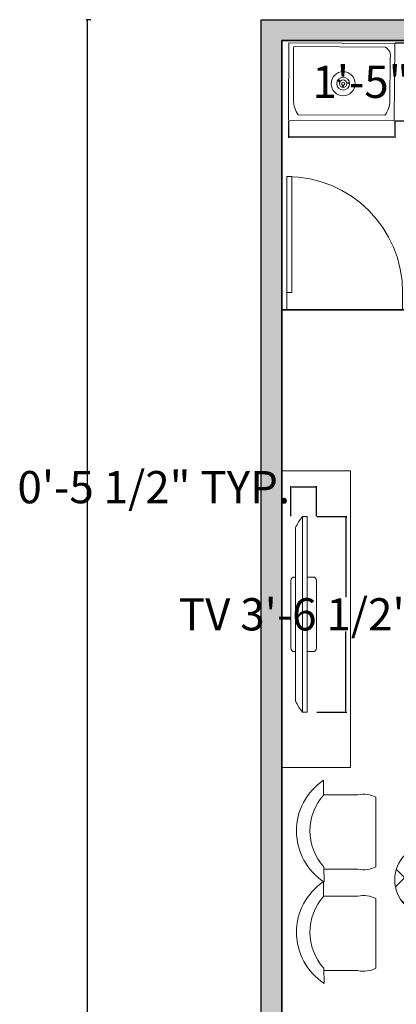
# Model space of a CAD drawing. Units: inches. Extents: x 0 to 4258, y 0 to 3769.
# Tile 20 of 30: x 3626 to 3708, y 3443 to 3657. Entities that reach past the tile are written whole.
import ezdxf

# ---------------------------------------------------------------- set-up
doc = ezdxf.new("R2010")
doc.units = ezdxf.units.IN
doc.header["$MEASUREMENT"] = 0
doc.layers.get('0').update_dxf_attribs({"color": 16})
for name, color, linetype, lineweight in [('A-ANNO-DIMS', 250, 'Continuous', 18), ('A-EQPM', 8, 'Continuous', 18), ('A-FLOR-FIXT', 250, 'Continuous', 18), ('A-WALL-PATT', 16, 'Continuous', 13), ('C-PROP', 150, 'Continuous', 25), ('doors', 250, 'Continuous', 18), ('furniture', 13, 'Continuous', 18), ('walls', 251, 'Continuous', 35)]:
    doc.layers.add(name, color=color, linetype=linetype, lineweight=lineweight)
doc.styles.get("Standard").update_dxf_attribs({"font": 'arial.ttf'})
doc.dimstyles.get("Standard").update_dxf_attribs({"dimtxt": 7, "dimasz": 0.18, "dimexe": 0.18, "dimexo": 0.0625, "dimgap": 0.09, "dimtad": 0, "dimtih": 1, "dimtoh": 1, "dimzin": 0, "dimdsep": 46, "dimlunit": 3, "dimtxsty": 'Standard', "dimcen": 0.09, "dimadec": 0, "dimazin": 0, "dimtfac": 1, "dimtofl": 0, "dimtmove": 0, "dimatfit": 3, "dimfxl": 1, "dimtolj": 1, "dimtzin": 0, "dimarcsym": 0})

# ---------------------------------------------------------------- blocks, each defined once
blk = doc.blocks.new('PLASMA-LARGE')
at = {"layer": 'furniture'}
for p, q in [((-7.26, 0), (7.26, 0)), ((-18.61, -1), (18.61, -1)), ((-8, -1), (-8, -0.74)), ((8, -1), (8, -0.74)), ((-21, -2.5), (21, -2.5)), ((-21, -2.5), (-21, -3.5)), ((-21, -3.5), (21, -3.5)), ((-8, -3.5), (-8, -4.76)), ((8, -3.5), (8, -4.76)), ((21, -2.5), (21, -3.5)), ((-7.26, -5.5), (7.26, -5.5))]:
    blk.add_line(p, q, dxfattribs=at)
for centre, radius, start, end in [((-7.26, -0.74), 0.744, 90, 180), ((7.26, -0.74), 0.744, 0, 90), ((-13.97, -11.05), 11.07, 114.7602, 129.4175), ((13.97, -11.05), 11.07, 50.5825, 65.2398), ((-7.26, -4.76), 0.744, 180, 270), ((7.26, -4.76), 0.744, 270, 0)]:
    blk.add_arc(centre, radius, start, end, dxfattribs=at)
blk = doc.blocks.new('*U23')
for p, q in [((0, 0), (0, -6)), ((40, 0), (40, -6))]:
    blk.add_line(p, q)
blk.add_lwpolyline([(0, 0), (0, 40), (1.75, 40), (1.75, 0)], close=True)
blk.add_arc((0, 0), 40, 0, 90)
blk = doc.blocks.new('*D25')
at = {"layer": 'A-ANNO-DIMS', "color": 0, "lineweight": -2, "transparency": 16777216}
for p, q in [((3641.78, 3656.79), (3640.81, 3656.79)), ((3640.99, 3656.61), (3640.99, 3300.46)), ((3640.99, 2936.97), (3640.99, 3293.13)), ((3641.78, 2936.79), (3640.81, 2936.79))]:
    blk.add_line(p, q, dxfattribs=at)
at = {"layer": 'A-ANNO-DIMS', "color": 0, "transparency": 16777216}
for points in [[(3640.96, 3656.61), (3641.02, 3656.61), (3640.99, 3656.79)], [(3640.96, 2936.97), (3641.02, 2936.97), (3640.99, 2936.79)]]:
    blk.add_solid(points, dxfattribs=at)
at = {"layer": 'Defpoints', "color": 0, "transparency": 16777216}
for p in [(3641.85, 3656.79), (3640.99, 2936.79), (3641.85, 2936.79)]:
    blk.add_point(p, dxfattribs=at)
at = {"layer": 'A-ANNO-DIMS', "color": 0, "transparency": 16777216, "insert": (3640.99, 3296.79), "char_height": 7, "attachment_point": 5}
blk.add_mtext("\\A1;60'", dxfattribs=at)
blk = doc.blocks.new('BASIN-RECTANGULAR')
for p, q in [((0.01, 1.29), (0.11, 17)), ((0.11, 17), (23.11, 16.85)), ((1.16, 16.16), (21.05, 16.03)), ((23.11, 16.85), (23, 0)), ((1.14, 13.79), (1.08, 4.5)), ((22.11, 13.65), (22.05, 4.36)), ((11.13, 8.4), (10.74, 8.87)), ((11.26, 8.61), (10.89, 9.05)), ((11.75, 7.78), (11.7, 7.3)), ((11.88, 7.27), (11.94, 7.76)), ((12.59, 8.3), (13.23, 8.41)), ((12.71, 8.08), (13.27, 8.19)), ((0, 0.15), (0.01, 1.29)), ((23, 0), (0, 0.15)), ((2.14, 1.35), (20.95, 1.23))]:
    blk.add_line(p, q)
for radius in [2.61, 1.39, 0.816, 0.338]:
    blk.add_circle((11.89, 8.09), radius)
for centre, radius, start, end in [((10.4, 14.91), 9.33, 172.3124, 186.9318), ((20.1, 14.18), 2.08, 345.2338, 62.9258), ((6.48, 4.56), 5.4, 180.6949, 216.4918), ((16.65, 4.5), 5.4, 322.7525, 358.5493)]:
    blk.add_arc(centre, radius, start, end)
blk = doc.blocks.new('SEATING-TWO-CHAIRS-AND-TABLE')
h = blk.add_hatch()
h.set_pattern_fill('AR-HBONE', color=256, angle=90)
h.set_pattern_definition([(135, (3403.542, -4056.0025), (-5.6568542, 3e-16), [12, -4]), (225, (3400.7137, -4053.174), (-5.6568542, 8e-16), [12, -4])])
h.paths.add_polyline_path([(7.59, 14.04, 1), (7.59, 29.23, 1)])
for p, q in [((30.53, 40.83), (30.5, 44.11)), ((19.25, 25.7), (19.25, 40.83)), ((23.18, 41.34), (30.53, 41.34)), ((23.18, 25.19), (30.53, 25.19)), ((30.63, 22.02), (30.63, 25.19)), ((30.53, 18.81), (30.5, 22.09)), ((23.18, 19.32), (30.53, 19.32)), ((19.25, 3.68), (19.25, 18.81)), ((23.18, 3.17), (30.53, 3.17)), ((30.63, 0), (30.63, 3.17))]:
    blk.add_line(p, q)
blk.add_circle((7.59, 21.64), 7.59)
for centre, radius, start, end in [((23.25, 33.02), 13.25, 303.8239, 56.829), ((21.94, 35.53), 5.94, 77.9198, 116.8624), ((22.13, 33.01), 11.48, 317.0375, 42.9625), ((21.94, 31), 5.94, 243.1376, 282.0802), ((23.25, 11.01), 13.25, 303.8239, 56.829), ((21.94, 13.51), 5.94, 77.9198, 116.8624), ((22.13, 10.99), 11.48, 317.0375, 42.9625), ((21.94, 8.98), 5.94, 243.1376, 282.0802)]:
    blk.add_arc(centre, radius, start, end)
blk = doc.blocks.new('TV-CONSOLE-CABINET')
for p, q in [((0, 0), (0, 64.44)), ((0, 64.44), (14.9, 64.44)), ((14.9, 0), (0, 0))]:
    blk.add_line(p, q)
blk = doc.blocks.new('*D36')
at = {"layer": 'A-ANNO-DIMS', "color": 0, "lineweight": -2, "transparency": 16777216}
for p, q in [((3690.88, 3548.93), (3697.37, 3548.93)), ((3697.19, 3548.75), (3697.19, 3531.4)), ((3697.19, 3506.63), (3697.19, 3523.98)), ((3690.88, 3506.45), (3697.37, 3506.45))]:
    blk.add_line(p, q, dxfattribs=at)
at = {"layer": 'A-ANNO-DIMS', "color": 0, "transparency": 16777216}
for points in [[(3697.16, 3548.75), (3697.22, 3548.75), (3697.19, 3548.93)], [(3697.16, 3506.63), (3697.22, 3506.63), (3697.19, 3506.45)]]:
    blk.add_solid(points, dxfattribs=at)
at = {"layer": 'Defpoints', "color": 0, "transparency": 16777216}
for p in [(3690.82, 3548.93), (3697.19, 3548.93), (3690.82, 3506.45)]:
    blk.add_point(p, dxfattribs=at)
at = {"layer": 'A-ANNO-DIMS', "color": 0, "transparency": 16777216, "insert": (3697.19, 3527.69), "char_height": 7, "attachment_point": 5}
blk.add_mtext('\\A1;TV 3\'-6 1/2" TYP.', dxfattribs=at)
blk = doc.blocks.new('*D37')
at = {"layer": 'A-ANNO-DIMS', "color": 0, "lineweight": -2, "transparency": 16777216}
for p, q in [((3685.25, 3555.3), (3685.07, 3555.3)), ((3685.25, 3548.99), (3685.25, 3555.48)), ((3690.64, 3555.3), (3685.43, 3555.3)), ((3690.82, 3548.99), (3690.82, 3555.48))]:
    blk.add_line(p, q, dxfattribs=at)
at = {"layer": 'A-ANNO-DIMS', "color": 0, "transparency": 16777216}
for points in [[(3685.43, 3555.33), (3685.43, 3555.27), (3685.25, 3555.3)], [(3690.64, 3555.33), (3690.64, 3555.27), (3690.82, 3555.3)]]:
    blk.add_solid(points, dxfattribs=at)
at = {"layer": 'Defpoints', "color": 0, "transparency": 16777216}
for p in [(3685.25, 3555.3), (3685.25, 3548.93), (3690.82, 3548.93)]:
    blk.add_point(p, dxfattribs=at)
at = {"layer": 'A-ANNO-DIMS', "color": 0, "transparency": 16777216, "insert": (3655.49, 3555.3), "char_height": 7, "attachment_point": 5}
blk.add_mtext('\\A1;0\'-5 1/2" TYP.', dxfattribs=at)
blk = doc.blocks.new('*D54')
at = {"layer": 'A-ANNO-DIMS', "color": 0, "lineweight": -2, "transparency": 16777216}
for p, q in [((3684.72, 3634.74), (3684.72, 3631.16)), ((3707.82, 3634.74), (3707.82, 3631.16)), ((3684.9, 3631.34), (3707.64, 3631.34)), ((3707.82, 3631.34), (3708, 3631.34))]:
    blk.add_line(p, q, dxfattribs=at)
at = {"layer": 'A-ANNO-DIMS', "color": 0, "transparency": 16777216}
for points in [[(3684.9, 3631.37), (3684.9, 3631.31), (3684.72, 3631.34)], [(3707.64, 3631.37), (3707.64, 3631.31), (3707.82, 3631.34)]]:
    blk.add_solid(points, dxfattribs=at)
at = {"layer": 'Defpoints', "color": 0, "transparency": 16777216}
for p in [(3684.72, 3634.8), (3707.82, 3634.8), (3707.82, 3631.34)]:
    blk.add_point(p, dxfattribs=at)
at = {"layer": 'A-ANNO-DIMS', "color": 0, "transparency": 16777216, "insert": (3748.02, 3631.34), "char_height": 7, "attachment_point": 5}
blk.add_mtext('\\A1;BASIN 1\'-11" TYP.', dxfattribs=at)
blk = doc.blocks.new('*D55')
at = {"layer": 'A-ANNO-DIMS', "color": 0, "lineweight": -2, "transparency": 16777216}
for p, q in [((3707.89, 3651.8), (3711.47, 3651.8)), ((3711.29, 3651.62), (3711.29, 3646.97)), ((3711.29, 3634.98), (3711.29, 3639.64)), ((3707.89, 3634.8), (3711.47, 3634.8))]:
    blk.add_line(p, q, dxfattribs=at)
at = {"layer": 'A-ANNO-DIMS', "color": 0, "transparency": 16777216}
for points in [[(3711.26, 3651.62), (3711.32, 3651.62), (3711.29, 3651.8)], [(3711.26, 3634.98), (3711.32, 3634.98), (3711.29, 3634.8)]]:
    blk.add_solid(points, dxfattribs=at)
at = {"layer": 'Defpoints', "color": 0, "transparency": 16777216}
for p in [(3707.82, 3651.8), (3711.29, 3651.8), (3707.82, 3634.8)]:
    blk.add_point(p, dxfattribs=at)
at = {"layer": 'A-ANNO-DIMS', "color": 0, "transparency": 16777216, "insert": (3711.29, 3643.3), "char_height": 7, "attachment_point": 5}
blk.add_mtext('\\A1;1\'-5" TYP.', dxfattribs=at)

msp = doc.modelspace()

# ---------------------------------------------------------------- hatches: boundary and pattern name
at = {"layer": 'A-WALL-PATT'}
h = msp.add_hatch(color=256, dxfattribs=at)
h.dxf.hatch_style = 1
h.paths.add_polyline_path([(3753.804, 3425.793), (3753.804, 3437.642), (3815.304, 3437.642), (3815.304, 3421.293), (3819.804, 3421.293), (3819.804, 3442.142), (3749.304, 3442.142), (3749.304, 3425.793), (3683.304, 3425.793), (3683.304, 3652.293), (3773.304, 3652.293), (3773.304, 3638.769), (3777.804, 3638.769), (3777.804, 3656.793), (3678.804, 3656.793), (3678.804, 3163.293), (3711.393, 3163.293), (3711.393, 3167.793), (3683.304, 3167.793), (3683.304, 3374.793), (3693.303, 3374.793), (3693.303, 3379.293), (3683.304, 3379.293), (3683.304, 3421.293), (3749.304, 3421.293), (3749.304, 3379.293), (3741.449, 3379.293), (3741.449, 3374.793), (3753.804, 3374.793)])

# ---------------------------------------------------------------- linework, layer by layer
at = {"layer": 'C-PROP'}
for p, q in [((3678.804, 3656.793), (4038.804, 3656.793)), ((3678.804, 2995.293), (3678.804, 3656.793))]:
    msp.add_line(p, q, dxfattribs=at)
at = {"layer": 'walls'}
for p, q in [((3683.304, 3652.293), (3773.304, 3652.293)), ((3683.304, 3425.793), (3683.304, 3652.293)), ((3683.304, 3593.793), (3815.304, 3593.793))]:
    msp.add_line(p, q, dxfattribs=at)

# ---------------------------------------------------------------- block references
at = {"layer": 'A-EQPM', "xscale": 1.011294184530666, "yscale": 1.011294184530666, "zscale": 1.011294184530666, "rotation": 89.99999999999999}
msp.add_blockref('PLASMA-LARGE', (3685.254, 3527.689), dxfattribs=at)
at = {"layer": 'A-FLOR-FIXT'}
msp.add_blockref('BASIN-RECTANGULAR', (3684.717, 3634.804), dxfattribs=at)
at = {"layer": 'doors', "xscale": 0.6294121846440242, "yscale": 0.6294121846440242, "zscale": 0.6294121846440242}
msp.add_blockref('*U23', (3684.348, 3597.57), dxfattribs=at)
at = {"layer": 'furniture', "rotation": 180}
for name, p in [('TV-CONSOLE-CABINET', (3698.2, 3558.871)), ('SEATING-TWO-CHAIRS-AND-TABLE', (3722.972, 3491.674))]:
    msp.add_blockref(name, p, dxfattribs=at)

# ---------------------------------------------------------------- dimensions: what is measured, and where the dimension line sits
at = {"layer": 'A-ANNO-DIMS'}
dim = msp.add_linear_dim(base=(3640.987, 2936.793), p1=(3641.847, 3656.793), p2=(3641.847, 2936.793), angle=90, dimstyle='Standard', override={"dimclrd": 0, "dimclre": 0, "dimclrt": 0}, dxfattribs=at)
dim.commit()
dim.dimension.update_dxf_attribs({"geometry": '*D25', "text_midpoint": (3640.987, 3296.793)})
for base, p1, p2, angle, text, picture, middle in [((3711.29, 3651.803), (3707.824, 3634.804), (3707.824, 3651.803), 90, '<> TYP.', '*D55', (3711.29, 3643.303)), ((3685.254, 3555.297), (3690.816, 3548.926), (3685.254, 3548.926), 180, '<> TYP.', '*D37', (3655.494, 3555.297)), ((3697.187, 3548.926), (3690.816, 3506.452), (3690.816, 3548.926), 90, 'TV <> TYP.', '*D36', (3697.187, 3527.689))]:
    dim = msp.add_linear_dim(base=base, p1=p1, p2=p2, angle=angle, text=text, dimstyle='Standard', override={"dimdec": 1, "dimlfac": 1, "dimrnd": 0, "dimzin": 1, "dimdsep": 46, "dimlunit": 4, "dimfrac": 2}, dxfattribs=at)
    dim.commit()
    dim.dimension.update_dxf_attribs({"geometry": picture, "text_midpoint": middle})
dim = msp.add_linear_dim(base=(3707.824, 3631.338), p1=(3684.717, 3634.804), p2=(3707.824, 3634.804), text='BASIN <> TYP.', dimstyle='Standard', override={"dimdec": 1, "dimlfac": 1, "dimrnd": 0, "dimzin": 1, "dimdsep": 46, "dimlunit": 4, "dimfrac": 2}, dxfattribs=at)
dim.commit()
dim.dimension.update_dxf_attribs({"geometry": '*D54', "text_midpoint": (3748.024, 3631.338)})

doc.saveas('drawing.dxf')
